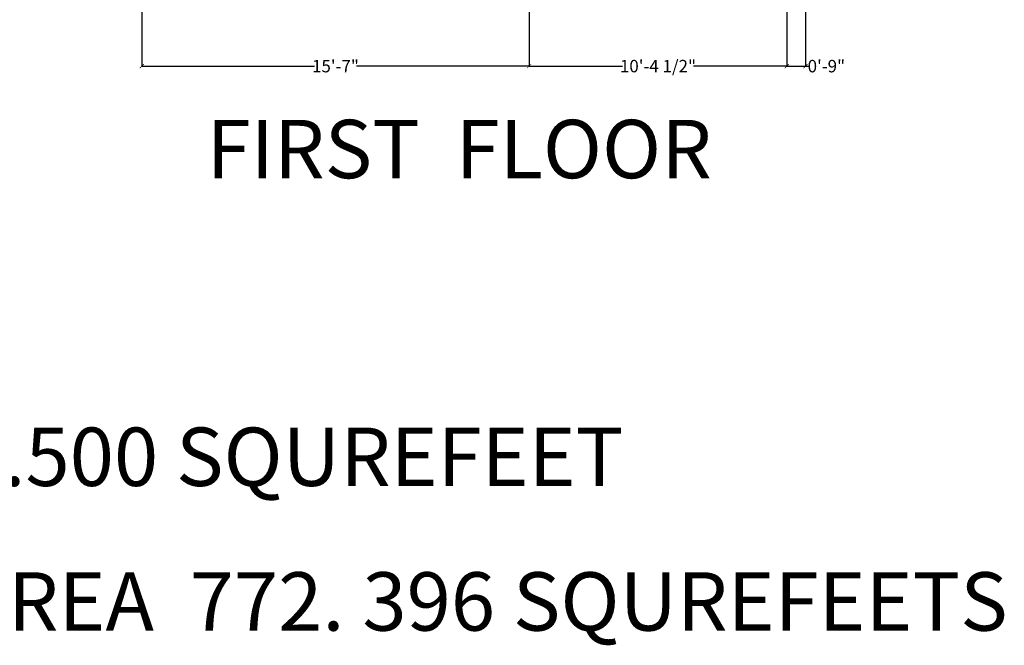
# Model space of a CAD drawing. Units: inches. Extents: x 528 to 2620, y -1066 to 798.
# Tile 20 of 41: x 966 to 1441, y -83 to 219. Entities that reach past the tile are written whole.
import ezdxf

# ---------------------------------------------------------------- set-up
doc = ezdxf.new("R2010")
doc.units = ezdxf.units.IN
doc.header["$MEASUREMENT"] = 0
doc.layers.add('A-ANNO-DIMS', color=2, linetype='Continuous', lineweight=18)
doc.layers.add('A-ANNO-TEXT', color=7, linetype='Continuous', lineweight=25)
doc.styles.get("Standard").update_dxf_attribs({"font": 'arial.ttf'})
doc.dimstyles.get("Standard").update_dxf_attribs({"dimtxt": 6, "dimasz": 2, "dimexe": 0.18, "dimexo": 0.0625, "dimgap": 0.09, "dimtad": 0, "dimtih": 1, "dimtoh": 1, "dimdec": 1, "dimzin": 0, "dimdsep": 46, "dimlunit": 3, "dimtxsty": 'Standard', "dimblk": 'ARCHTICK', "dimcen": 0.09, "dimadec": 0, "dimazin": 0, "dimtfac": 1, "dimtdec": 1, "dimtofl": 0, "dimtmove": 0, "dimatfit": 3, "dimfxl": 1, "dimtolj": 1, "dimtzin": 0, "dimarcsym": 0})

# ---------------------------------------------------------------- blocks, each defined once
blk = doc.blocks.new('_ArchTick')
at = {"color": 0, "linetype": 'ByBlock', "const_width": 0.15}
blk.add_lwpolyline([(-0.5, -0.5), (0.5, 0.5)], dxfattribs=at)
blk = doc.blocks.new('*D60')
at = {"layer": 'A-ANNO-DIMS', "color": 0, "lineweight": -2, "transparency": 16777216}
for p, q in [((1024.5, 228.36), (1024.5, 196.24)), ((1211.5, 228.36), (1211.5, 196.24)), ((1024.5, 196.42), (1107.88, 196.42)), ((1211.5, 196.42), (1128.11, 196.42))]:
    blk.add_line(p, q, dxfattribs=at)
at = {"layer": 'Defpoints', "color": 0, "transparency": 16777216}
for p in [(1024.5, 228.42), (1211.5, 228.42), (1211.5, 196.42)]:
    blk.add_point(p, dxfattribs=at)
at = {"layer": 'A-ANNO-DIMS', "color": 0, "lineweight": -2, "transparency": 16777216, "xscale": 2, "yscale": 2, "zscale": 2, "rotation": 180}
blk.add_blockref('_ArchTick', (1024.5, 196.42), dxfattribs=at)
at = {"layer": 'A-ANNO-DIMS', "color": 0, "lineweight": -2, "transparency": 16777216, "xscale": 2, "yscale": 2, "zscale": 2}
blk.add_blockref('_ArchTick', (1211.5, 196.42), dxfattribs=at)
at = {"layer": 'A-ANNO-DIMS', "color": 0, "transparency": 16777216, "insert": (1118, 196.42), "char_height": 6, "attachment_point": 5}
blk.add_mtext('\\A1;15\'-7"', dxfattribs=at)
blk = doc.blocks.new('*D61')
at = {"layer": 'A-ANNO-DIMS', "color": 0, "lineweight": -2, "transparency": 16777216}
for p, q in [((1336, 277.86), (1336, 196.24)), ((1211.5, 228.36), (1211.5, 196.24)), ((1211.5, 196.42), (1256.64, 196.42)), ((1336, 196.42), (1290.85, 196.42))]:
    blk.add_line(p, q, dxfattribs=at)
at = {"layer": 'Defpoints', "color": 0, "transparency": 16777216}
for p in [(1336, 277.92), (1211.5, 228.42), (1336, 196.42)]:
    blk.add_point(p, dxfattribs=at)
at = {"layer": 'A-ANNO-DIMS', "color": 0, "lineweight": -2, "transparency": 16777216, "xscale": 2, "yscale": 2, "zscale": 2, "rotation": 180}
blk.add_blockref('_ArchTick', (1211.5, 196.42), dxfattribs=at)
at = {"layer": 'A-ANNO-DIMS', "color": 0, "lineweight": -2, "transparency": 16777216, "xscale": 2, "yscale": 2, "zscale": 2}
blk.add_blockref('_ArchTick', (1336, 196.42), dxfattribs=at)
at = {"layer": 'A-ANNO-DIMS', "color": 0, "transparency": 16777216, "insert": (1273.75, 196.42), "char_height": 6, "attachment_point": 5}
blk.add_mtext('\\A1;10\'-4 1/2"', dxfattribs=at)
blk = doc.blocks.new('*D62')
at = {"layer": 'A-ANNO-DIMS', "color": 0, "lineweight": -2, "transparency": 16777216}
for p, q in [((1336, 277.86), (1336, 196.24)), ((1345, 268.86), (1345, 196.24)), ((1336, 196.42), (1345, 196.42)), ((1345, 196.42), (1347, 196.42))]:
    blk.add_line(p, q, dxfattribs=at)
at = {"layer": 'Defpoints', "color": 0, "transparency": 16777216}
for p in [(1336, 277.92), (1345, 268.92), (1345, 196.42)]:
    blk.add_point(p, dxfattribs=at)
at = {"layer": 'A-ANNO-DIMS', "color": 0, "lineweight": -2, "transparency": 16777216, "xscale": 2, "yscale": 2, "zscale": 2, "rotation": 180}
blk.add_blockref('_ArchTick', (1336, 196.42), dxfattribs=at)
at = {"layer": 'A-ANNO-DIMS', "color": 0, "lineweight": -2, "transparency": 16777216, "xscale": 2, "yscale": 2, "zscale": 2}
blk.add_blockref('_ArchTick', (1345, 196.42), dxfattribs=at)
at = {"layer": 'A-ANNO-DIMS', "color": 0, "transparency": 16777216, "insert": (1355.06, 196.42), "char_height": 6, "attachment_point": 5}
blk.add_mtext('\\A1;0\'-9"', dxfattribs=at)

msp = doc.modelspace()

# ---------------------------------------------------------------- texts
at = {"layer": 'A-ANNO-TEXT'}
for s, p in [('FIRST  FLOOR', (1055.82, 142.26)), ('TOTAL AREA  1362.500 SQUREFEET', (633.4, -6.41)), ('CONSTRUCTION AREA  772. 396 SQUREFEETS', (633.4, -76.3))]:
    msp.add_text(s, height=28.2129, dxfattribs=at).set_placement(p)

# ---------------------------------------------------------------- dimensions: what is measured, and where the dimension line sits
at = {"layer": 'A-ANNO-DIMS'}
for base, p1, p2, picture, middle in [((1336, 196.42), (1211.5, 228.42), (1336, 277.92), '*D61', (1273.75, 196.42)), ((1345, 196.42), (1336, 277.92), (1345, 268.92), '*D62', (1355.06, 196.42)), ((1211.5, 196.42), (1024.5, 228.42), (1211.5, 228.42), '*D60', (1118, 196.42))]:
    dim = msp.add_linear_dim(base=base, p1=p1, p2=p2, dimstyle='Standard', override={"dimdec": 1, "dimlfac": 1, "dimrnd": 0, "dimzin": 1, "dimdsep": 46, "dimlunit": 4, "dimfrac": 2}, dxfattribs=at)
    dim.commit()
    dim.dimension.update_dxf_attribs({"geometry": picture, "text_midpoint": middle})

doc.saveas('drawing.dxf')
